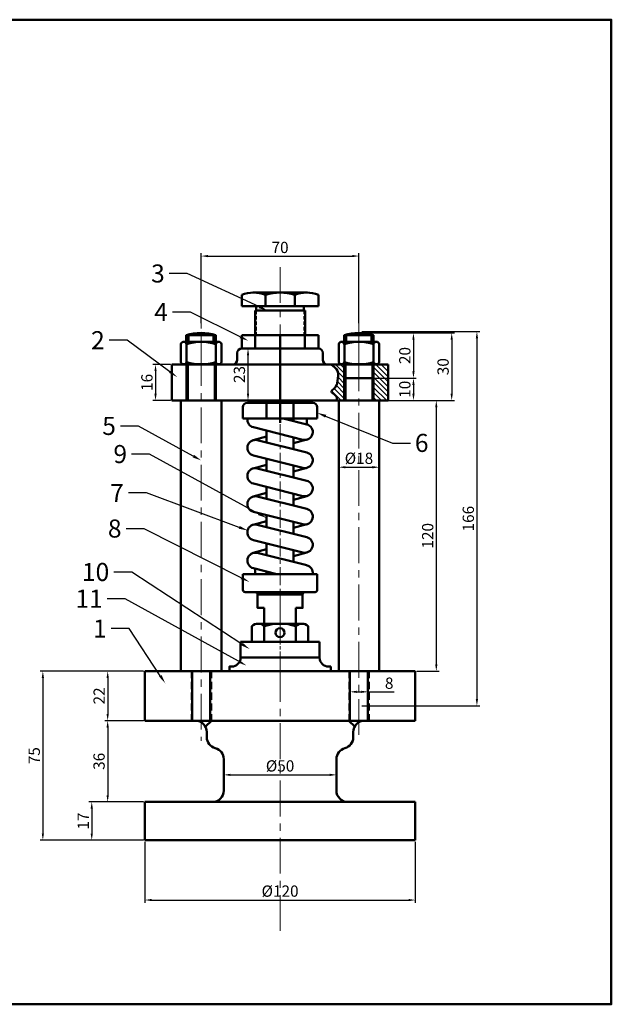
# Model space of a CAD drawing. Units: millimetres. Extents: x -656 to 85, y 134 to 571.
# Tile 5 of 5: x -178 to 85, y 134 to 571. Entities that reach past the tile are written whole.
import ezdxf
from ezdxf import colors
from ezdxf.entities.mleader import LeaderData, LeaderLine
from ezdxf.math import Vec2, Vec3

# ---------------------------------------------------------------- set-up
doc = ezdxf.new("R2010")
doc.units = ezdxf.units.MM
doc.header["$LTSCALE"] = 0.5
doc.linetypes.add('CENTER', pattern=[50.8, 31.75, -6.35, 6.35, -6.35])
doc.linetypes.add('HIDDEN', pattern=[9.525, 6.35, -3.175])
for name, color, linetype, lineweight in [('M-CNTR', 1, 'CENTER', 18), ('M-DIMS', 2, 'Continuous', 25), ('M-HATC', 8, 'Continuous', 18), ('M-HIDN', 3, 'HIDDEN', 25), ('M-OUTL', 7, 'Continuous', 50), ('M-TEXT', 7, 'Continuous', 25), ('M-TTLB', 7, 'Continuous', 50)]:
    doc.layers.add(name, color=color, linetype=linetype, lineweight=lineweight)
doc.styles.get("Standard").update_dxf_attribs({"font": 'arial.ttf'})
doc.dimstyles.new('ISO-25', dxfattribs={"dimtxt": 5, "dimasz": 3, "dimexe": 1.25, "dimexo": 0.625, "dimtad": 1, "dimtoh": 1, "dimdec": 0, "dimtxsty": 'Standard', "dimcen": 2.5, "dimadec": 0, "dimazin": 0, "dimtfac": 1, "dimtdec": 0, "dimtofl": 0, "dimtmove": 0, "dimatfit": 3, "dimfxl": 1, "dimarcsym": 0})

# ---------------------------------------------------------------- blocks, each defined once
blk = doc.blocks.new('*U82')
at = {"layer": 'M-CNTR', "color": 0, "transparency": 16777216}
blk.add_line((0, -16.59), (0, 25.52), dxfattribs=at)
blk = doc.blocks.new('*U83')
at = {"layer": 'M-CNTR', "color": 0, "transparency": 16777216}
blk.add_line((0, -7.5), (0, 12.59), dxfattribs=at)
blk = doc.blocks.new('*U84')
at = {"layer": 'M-CNTR', "color": 0, "transparency": 16777216}
blk.add_line((0, -7.5), (0, 12.59), dxfattribs=at)
blk = doc.blocks.new('*D85')
at = {"layer": 'Defpoints', "color": 0, "ltscale": 0.5, "transparency": 16777216}
for p in [(-122.34, 207.21), (-2.34, 207.21), (-2.34, 180.72)]:
    blk.add_point(p, dxfattribs=at)
at = {"layer": 'M-DIMS', "color": 0, "lineweight": -2, "ltscale": 0.5, "transparency": 16777216}
for p, q in [((-122.34, 206.59), (-122.34, 179.47)), ((-2.34, 206.59), (-2.34, 179.47)), ((-119.34, 180.72), (-5.34, 180.72))]:
    blk.add_line(p, q, dxfattribs=at)
at = {"layer": 'M-DIMS', "color": 0, "ltscale": 0.5, "transparency": 16777216}
for points in [[(-119.34, 181.22), (-119.34, 180.22), (-122.34, 180.72)], [(-5.34, 181.22), (-5.34, 180.22), (-2.34, 180.72)]]:
    blk.add_solid(points, dxfattribs=at)
at = {"layer": 'M-DIMS', "color": 0, "ltscale": 0.5, "transparency": 16777216, "insert": (-62.34, 184.03), "char_height": 5, "attachment_point": 5}
blk.add_mtext('%%C120', dxfattribs=at)
blk = doc.blocks.new('*D86')
at = {"layer": 'Defpoints', "color": 0, "ltscale": 0.5, "transparency": 16777216}
for p in [(-122.34, 282.21), (-167.59, 207.21), (-122.34, 207.21)]:
    blk.add_point(p, dxfattribs=at)
at = {"layer": 'M-DIMS', "color": 0, "lineweight": -2, "ltscale": 0.5, "transparency": 16777216}
for p, q in [((-122.96, 282.21), (-168.84, 282.21)), ((-167.59, 279.21), (-167.59, 210.21)), ((-122.96, 207.21), (-168.84, 207.21))]:
    blk.add_line(p, q, dxfattribs=at)
at = {"layer": 'M-DIMS', "color": 0, "ltscale": 0.5, "transparency": 16777216}
for points in [[(-168.09, 279.21), (-167.09, 279.21), (-167.59, 282.21)], [(-168.09, 210.21), (-167.09, 210.21), (-167.59, 207.21)]]:
    blk.add_solid(points, dxfattribs=at)
at = {"layer": 'M-DIMS', "color": 0, "ltscale": 0.5, "transparency": 16777216, "insert": (-170.76, 244.71), "char_height": 5, "attachment_point": 5, "rotation": 90}
blk.add_mtext('75', dxfattribs=at)
blk = doc.blocks.new('*D87')
at = {"layer": 'Defpoints', "color": 0, "ltscale": 0.5, "transparency": 16777216}
for p in [(-122.34, 282.21), (-138.83, 260.21), (-122.34, 260.21)]:
    blk.add_point(p, dxfattribs=at)
at = {"layer": 'M-DIMS', "color": 0, "lineweight": -2, "ltscale": 0.5, "transparency": 16777216}
for p, q in [((-122.96, 282.21), (-140.08, 282.21)), ((-138.83, 279.21), (-138.83, 263.21)), ((-122.96, 260.21), (-140.08, 260.21))]:
    blk.add_line(p, q, dxfattribs=at)
at = {"layer": 'M-DIMS', "color": 0, "ltscale": 0.5, "transparency": 16777216}
for points in [[(-139.33, 279.21), (-138.33, 279.21), (-138.83, 282.21)], [(-139.33, 263.21), (-138.33, 263.21), (-138.83, 260.21)]]:
    blk.add_solid(points, dxfattribs=at)
at = {"layer": 'M-DIMS', "color": 0, "ltscale": 0.5, "transparency": 16777216, "insert": (-141.97, 271.21), "char_height": 5, "attachment_point": 5, "rotation": 90}
blk.add_mtext('22', dxfattribs=at)
blk = doc.blocks.new('*D88')
at = {"layer": 'Defpoints', "color": 0, "ltscale": 0.5, "transparency": 16777216}
for p in [(-122.34, 224.21), (-145.9, 207.21), (-122.34, 207.21)]:
    blk.add_point(p, dxfattribs=at)
at = {"layer": 'M-DIMS', "color": 0, "lineweight": -2, "ltscale": 0.5, "transparency": 16777216}
for p, q in [((-122.96, 224.21), (-147.15, 224.21)), ((-145.9, 221.21), (-145.9, 210.21)), ((-122.96, 207.21), (-147.15, 207.21))]:
    blk.add_line(p, q, dxfattribs=at)
at = {"layer": 'M-DIMS', "color": 0, "ltscale": 0.5, "transparency": 16777216}
for points in [[(-146.4, 221.21), (-145.4, 221.21), (-145.9, 224.21)], [(-146.4, 210.21), (-145.4, 210.21), (-145.9, 207.21)]]:
    blk.add_solid(points, dxfattribs=at)
at = {"layer": 'M-DIMS', "color": 0, "ltscale": 0.5, "transparency": 16777216, "insert": (-149.04, 215.71), "char_height": 5, "attachment_point": 5, "rotation": 90}
blk.add_mtext('17', dxfattribs=at)
blk = doc.blocks.new('*D89')
at = {"layer": 'Defpoints', "color": 0, "ltscale": 0.5, "transparency": 16777216}
for p in [(-122.34, 260.21), (-138.83, 224.21), (-122.34, 224.21)]:
    blk.add_point(p, dxfattribs=at)
at = {"layer": 'M-DIMS', "color": 0, "lineweight": -2, "ltscale": 0.5, "transparency": 16777216}
for p, q in [((-122.96, 260.21), (-140.08, 260.21)), ((-138.83, 257.21), (-138.83, 227.21)), ((-122.96, 224.21), (-140.08, 224.21))]:
    blk.add_line(p, q, dxfattribs=at)
at = {"layer": 'M-DIMS', "color": 0, "ltscale": 0.5, "transparency": 16777216}
for points in [[(-139.33, 257.21), (-138.33, 257.21), (-138.83, 260.21)], [(-139.33, 227.21), (-138.33, 227.21), (-138.83, 224.21)]]:
    blk.add_solid(points, dxfattribs=at)
at = {"layer": 'M-DIMS', "color": 0, "ltscale": 0.5, "transparency": 16777216, "insert": (-142.01, 242.21), "char_height": 5, "attachment_point": 5, "rotation": 90}
blk.add_mtext('36', dxfattribs=at)
blk = doc.blocks.new('*D90')
at = {"layer": 'Defpoints', "color": 0, "ltscale": 0.5, "transparency": 16777216}
for p in [(-87.34, 236.21), (-37.34, 236.21), (-37.34, 236.21)]:
    blk.add_point(p, dxfattribs=at)
at = {"layer": 'M-DIMS', "color": 0, "lineweight": -2, "ltscale": 0.5, "transparency": 16777216}
for p, q in [((-87.34, 236.84), (-87.34, 237.46)), ((-84.34, 236.21), (-40.34, 236.21)), ((-37.34, 236.84), (-37.34, 237.46))]:
    blk.add_line(p, q, dxfattribs=at)
at = {"layer": 'M-DIMS', "color": 0, "ltscale": 0.5, "transparency": 16777216}
for points in [[(-84.34, 236.71), (-84.34, 235.71), (-87.34, 236.21)], [(-40.34, 236.71), (-40.34, 235.71), (-37.34, 236.21)]]:
    blk.add_solid(points, dxfattribs=at)
at = {"layer": 'M-DIMS', "color": 0, "ltscale": 0.5, "transparency": 16777216, "insert": (-62.34, 239.53), "char_height": 5, "attachment_point": 5}
blk.add_mtext('%%C50', dxfattribs=at)
blk = doc.blocks.new('*D91')
at = {"layer": 'Defpoints', "color": 0, "ltscale": 0.5, "transparency": 16777216}
for p in [(-31.34, 271.21), (-23.34, 273.03), (-23.34, 271.21)]:
    blk.add_point(p, dxfattribs=at)
at = {"layer": 'M-DIMS', "color": 0, "lineweight": -2, "ltscale": 0.5, "transparency": 16777216}
for p, q in [((-31.34, 271.84), (-31.34, 274.28)), ((-28.34, 273.03), (-26.34, 273.03)), ((-23.34, 271.84), (-23.34, 274.28)), ((-23.34, 273.03), (-11.66, 273.03))]:
    blk.add_line(p, q, dxfattribs=at)
at = {"layer": 'M-DIMS', "color": 0, "ltscale": 0.5, "transparency": 16777216}
for points in [[(-28.34, 273.53), (-28.34, 272.53), (-31.34, 273.03)], [(-26.34, 273.53), (-26.34, 272.53), (-23.34, 273.03)]]:
    blk.add_solid(points, dxfattribs=at)
at = {"layer": 'M-DIMS', "color": 0, "ltscale": 0.5, "transparency": 16777216, "insert": (-13.93, 276.21), "char_height": 5, "attachment_point": 5}
blk.add_mtext('8', dxfattribs=at)
blk = doc.blocks.new('*D92')
at = {"layer": 'Defpoints', "color": 0, "ltscale": 0.5, "transparency": 16777216}
for p in [(-26.71, 432.8), (-26.71, 266.8), (25, 266.8)]:
    blk.add_point(p, dxfattribs=at)
at = {"layer": 'M-DIMS', "color": 0, "lineweight": -2, "ltscale": 0.5, "transparency": 16777216}
for p, q in [((-26.09, 432.8), (26.25, 432.8)), ((25, 429.8), (25, 269.8)), ((-26.09, 266.8), (26.25, 266.8))]:
    blk.add_line(p, q, dxfattribs=at)
at = {"layer": 'M-DIMS', "color": 0, "ltscale": 0.5, "transparency": 16777216}
for points in [[(24.5, 429.8), (25.5, 429.8), (25, 432.8)], [(24.5, 269.8), (25.5, 269.8), (25, 266.8)]]:
    blk.add_solid(points, dxfattribs=at)
at = {"layer": 'M-DIMS', "color": 0, "ltscale": 0.5, "transparency": 16777216, "insert": (21.82, 349.8), "char_height": 5, "attachment_point": 5, "rotation": 90}
blk.add_mtext('166', dxfattribs=at)
blk = doc.blocks.new('*D93')
at = {"layer": 'Defpoints', "color": 0, "ltscale": 0.5, "transparency": 16777216}
for p in [(-27.4, 432.12), (-27.34, 402.21), (13.81, 402.21)]:
    blk.add_point(p, dxfattribs=at)
at = {"layer": 'M-DIMS', "color": 0, "lineweight": -2, "ltscale": 0.5, "transparency": 16777216}
for p, q in [((-26.77, 432.12), (15.06, 432.12)), ((13.81, 429.12), (13.81, 405.21)), ((-26.71, 402.21), (15.06, 402.21))]:
    blk.add_line(p, q, dxfattribs=at)
at = {"layer": 'M-DIMS', "color": 0, "ltscale": 0.5, "transparency": 16777216}
for points in [[(13.31, 429.12), (14.31, 429.12), (13.81, 432.12)], [(13.31, 405.21), (14.31, 405.21), (13.81, 402.21)]]:
    blk.add_solid(points, dxfattribs=at)
at = {"layer": 'M-DIMS', "color": 0, "ltscale": 0.5, "transparency": 16777216, "insert": (10.63, 417.17), "char_height": 5, "attachment_point": 5, "rotation": 90}
blk.add_mtext('30', dxfattribs=at)
blk = doc.blocks.new('*D94')
at = {"layer": 'Defpoints', "color": 0, "ltscale": 0.5, "transparency": 16777216}
for p in [(-27.34, 432.12), (-27.34, 412.12), (-3.16, 412.12)]:
    blk.add_point(p, dxfattribs=at)
at = {"layer": 'M-DIMS', "color": 0, "lineweight": -2, "ltscale": 0.5, "transparency": 16777216}
for p, q in [((-26.71, 432.12), (-1.91, 432.12)), ((-3.16, 429.12), (-3.16, 415.12)), ((-26.71, 412.12), (-1.91, 412.12))]:
    blk.add_line(p, q, dxfattribs=at)
at = {"layer": 'M-DIMS', "color": 0, "ltscale": 0.5, "transparency": 16777216}
for points in [[(-3.66, 429.12), (-2.66, 429.12), (-3.16, 432.12)], [(-3.66, 415.12), (-2.66, 415.12), (-3.16, 412.12)]]:
    blk.add_solid(points, dxfattribs=at)
at = {"layer": 'M-DIMS', "color": 0, "ltscale": 0.5, "transparency": 16777216, "insert": (-6.34, 422.12), "char_height": 5, "attachment_point": 5, "rotation": 90}
blk.add_mtext('20', dxfattribs=at)
blk = doc.blocks.new('*D95')
at = {"layer": 'Defpoints', "color": 0, "ltscale": 0.5, "transparency": 16777216}
for p in [(-11.41, 412.12), (-11.41, 402.21), (-3.16, 402.21)]:
    blk.add_point(p, dxfattribs=at)
at = {"layer": 'M-DIMS', "color": 0, "lineweight": -2, "ltscale": 0.5, "transparency": 16777216}
for p, q in [((-10.78, 412.12), (-1.91, 412.12)), ((-3.16, 409.12), (-3.16, 405.21)), ((-10.78, 402.21), (-1.91, 402.21))]:
    blk.add_line(p, q, dxfattribs=at)
at = {"layer": 'M-DIMS', "color": 0, "ltscale": 0.5, "transparency": 16777216}
for points in [[(-3.66, 409.12), (-2.66, 409.12), (-3.16, 412.12)], [(-3.66, 405.21), (-2.66, 405.21), (-3.16, 402.21)]]:
    blk.add_solid(points, dxfattribs=at)
at = {"layer": 'M-DIMS', "color": 0, "ltscale": 0.5, "transparency": 16777216, "insert": (-6.34, 407.17), "char_height": 5, "attachment_point": 5, "rotation": 90}
blk.add_mtext('10', dxfattribs=at)
blk = doc.blocks.new('*D96')
at = {"layer": 'Defpoints', "color": 0, "ltscale": 0.5, "transparency": 16777216}
for p in [(-36.34, 372.6), (-18.34, 372.6), (-18.34, 372.6)]:
    blk.add_point(p, dxfattribs=at)
at = {"layer": 'M-DIMS', "color": 0, "lineweight": -2, "ltscale": 0.5, "transparency": 16777216}
for p, q in [((-36.34, 373.23), (-36.34, 373.85)), ((-33.34, 372.6), (-21.34, 372.6)), ((-18.34, 373.23), (-18.34, 373.85))]:
    blk.add_line(p, q, dxfattribs=at)
at = {"layer": 'M-DIMS', "color": 0, "ltscale": 0.5, "transparency": 16777216}
for points in [[(-33.34, 373.1), (-33.34, 372.1), (-36.34, 372.6)], [(-21.34, 373.1), (-21.34, 372.1), (-18.34, 372.6)]]:
    blk.add_solid(points, dxfattribs=at)
at = {"layer": 'M-DIMS', "color": 0, "ltscale": 0.5, "transparency": 16777216, "insert": (-27.34, 375.92), "char_height": 5, "attachment_point": 5}
blk.add_mtext('%%C18', dxfattribs=at)
blk = doc.blocks.new('*D97')
at = {"layer": 'Defpoints', "color": 0, "ltscale": 0.5, "transparency": 16777216}
for p in [(1.86, 402.21), (-2.34, 282.21), (6.97, 282.21)]:
    blk.add_point(p, dxfattribs=at)
at = {"layer": 'M-DIMS', "color": 0, "lineweight": -2, "ltscale": 0.5, "transparency": 16777216}
for p, q in [((2.49, 402.21), (8.22, 402.21)), ((6.97, 399.21), (6.97, 285.21)), ((-1.71, 282.21), (8.22, 282.21))]:
    blk.add_line(p, q, dxfattribs=at)
at = {"layer": 'M-DIMS', "color": 0, "ltscale": 0.5, "transparency": 16777216}
for points in [[(6.47, 399.21), (7.47, 399.21), (6.97, 402.21)], [(6.47, 285.21), (7.47, 285.21), (6.97, 282.21)]]:
    blk.add_solid(points, dxfattribs=at)
at = {"layer": 'M-DIMS', "color": 0, "ltscale": 0.5, "transparency": 16777216, "insert": (3.8, 342.21), "char_height": 5, "attachment_point": 5, "rotation": 90}
blk.add_mtext('120', dxfattribs=at)
blk = doc.blocks.new('*D98')
at = {"layer": 'Defpoints', "color": 0, "ltscale": 0.5, "transparency": 16777216}
for p in [(-110.34, 418.21), (-117.6, 402.21), (-110.34, 402.21)]:
    blk.add_point(p, dxfattribs=at)
at = {"layer": 'M-DIMS', "color": 0, "lineweight": -2, "ltscale": 0.5, "transparency": 16777216}
for p, q in [((-110.96, 418.21), (-118.85, 418.21)), ((-117.6, 415.21), (-117.6, 405.21)), ((-110.96, 402.21), (-118.85, 402.21))]:
    blk.add_line(p, q, dxfattribs=at)
at = {"layer": 'M-DIMS', "color": 0, "ltscale": 0.5, "transparency": 16777216}
for points in [[(-118.1, 415.21), (-117.1, 415.21), (-117.6, 418.21)], [(-118.1, 405.21), (-117.1, 405.21), (-117.6, 402.21)]]:
    blk.add_solid(points, dxfattribs=at)
at = {"layer": 'M-DIMS', "color": 0, "ltscale": 0.5, "transparency": 16777216, "insert": (-120.78, 410.21), "char_height": 5, "attachment_point": 5, "rotation": 90}
blk.add_mtext('16', dxfattribs=at)
blk = doc.blocks.new('*D99')
at = {"layer": 'Defpoints', "color": 0, "ltscale": 0.5, "transparency": 16777216}
for p in [(-27.34, 466.22), (-97.34, 435.8), (-27.34, 435.8)]:
    blk.add_point(p, dxfattribs=at)
at = {"layer": 'M-DIMS', "color": 0, "lineweight": -2, "ltscale": 0.5, "transparency": 16777216}
for p, q in [((-97.34, 436.43), (-97.34, 467.47)), ((-27.34, 436.43), (-27.34, 467.47)), ((-94.34, 466.22), (-30.34, 466.22))]:
    blk.add_line(p, q, dxfattribs=at)
at = {"layer": 'M-DIMS', "color": 0, "ltscale": 0.5, "transparency": 16777216}
for points in [[(-94.34, 466.72), (-94.34, 465.72), (-97.34, 466.22)], [(-30.34, 466.72), (-30.34, 465.72), (-27.34, 466.22)]]:
    blk.add_solid(points, dxfattribs=at)
at = {"layer": 'M-DIMS', "color": 0, "ltscale": 0.5, "transparency": 16777216, "insert": (-62.34, 469.4), "char_height": 5, "attachment_point": 5}
blk.add_mtext('70', dxfattribs=at)
blk = doc.blocks.new('*D100')
at = {"layer": 'Defpoints', "color": 0, "ltscale": 0.5, "transparency": 16777216}
for p in [(-76.68, 425.21), (-76.56, 425.21), (-76.68, 402.21)]:
    blk.add_point(p, dxfattribs=at)
at = {"layer": 'M-DIMS', "color": 0, "lineweight": -2, "ltscale": 0.5, "transparency": 16777216}
for p, q in [((-76.06, 425.21), (-75.31, 425.21)), ((-76.56, 405.21), (-76.56, 422.21)), ((-76.06, 402.21), (-75.31, 402.21))]:
    blk.add_line(p, q, dxfattribs=at)
at = {"layer": 'M-DIMS', "color": 0, "ltscale": 0.5, "transparency": 16777216}
for points in [[(-77.06, 422.21), (-76.06, 422.21), (-76.56, 425.21)], [(-77.06, 405.21), (-76.06, 405.21), (-76.56, 402.21)]]:
    blk.add_solid(points, dxfattribs=at)
at = {"layer": 'M-DIMS', "color": 0, "ltscale": 0.5, "transparency": 16777216, "insert": (-79.74, 413.71), "char_height": 5, "attachment_point": 5, "rotation": 90}
blk.add_mtext('23', dxfattribs=at)
blk = doc.blocks.new('NUT-HEX-LOCK')
at = {"ltscale": 0.5}
for p, q in [((38.72, -408.22), (38.72, -405.22)), ((51.84, -405.22), (38.72, -405.22)), ((51.84, -408.22), (51.84, -405.22)), ((36.34, -409.22), (36.34, -417.22)), ((38.84, -409.22), (38.84, -417.22)), ((51.84, -417.22), (51.84, -409.22)), ((54.34, -417.22), (54.34, -409.22))]:
    blk.add_line(p, q, dxfattribs=at)
for centre, radius, start, end in [((45.28, -428.53), 24.22, 74.2897, 105.7103), ((37.59, -409.5), 1.28, 12.6787, 167.3213), ((45.34, -429.84), 21.62, 72.5077, 107.4923), ((53.09, -409.5), 1.28, 12.6782, 167.3218), ((37.59, -416.93), 1.28, 192.6787, 347.3213), ((45.34, -396.59), 21.62, 252.5077, 287.4923), ((53.09, -416.93), 1.28, 192.6782, 347.3218)]:
    blk.add_arc(centre, radius, start, end, dxfattribs=at)
blk = doc.blocks.new('STUD-ROD')
at = {"ltscale": 0.5}
for p, q in [((0, 120), (0, 0)), ((18, 120), (0, 120)), ((18, 0), (18, 120)), ((0, 0), (18, 0))]:
    blk.add_line(p, q, dxfattribs=at)

msp = doc.modelspace()

# ---------------------------------------------------------------- hatches: boundary and pattern name
at = {"layer": 'M-HATC', "ltscale": 0.5}
h = msp.add_hatch(dxfattribs=at)
h.set_pattern_fill('ANSI31', color=256, scale=0.5, angle=90)
h.set_pattern_definition([(135, (-1832.0751, -452.3756), (-1.122532, -1.122532), [])])
h.paths.add_polyline_path([(-14.34, 418.21), (-20.84, 418.21), (-20.84, 402.21), (-18.34, 402.21), (-14.34, 402.21)])
edge = h.paths.add_edge_path()
edge.add_line((-33.84, 418.21), (-35.1, 418.21))
edge.add_line((-35.1, 418.21), (-39.78, 418.21))
edge.add_spline(control_points=[(-39.78, 418.21), (-38.56, 417.35), (-36.05, 415.56), (-36.85, 411.09), (-37.28, 407.9), (-40.74, 405.9), (-37.02, 404.71), (-37.01, 402.69), (-37.37, 402.21)], knot_values=[0, 0, 0, 0, 4.136966, 8.535604, 12.069689, 14.056123, 17.152579, 18.950395, 18.950395, 18.950395, 18.950395], degree=3, periodic=0)
edge.add_line((-37.37, 402.21), (-33.84, 402.21))
edge.add_line((-33.84, 402.21), (-33.84, 418.21))

# ---------------------------------------------------------------- linework, layer by layer
at = {"layer": 'M-CNTR'}
for p, q in [((-97.34, 449.93), (-97.34, 251.34)), ((-27.34, 447.57), (-27.34, 252.71)), ((-62.34, 167.01), (-62.34, 307.88))]:
    msp.add_line(p, q, dxfattribs=at)
at = {"layer": 'M-CNTR', "ltscale": 0.5}
msp.add_line((-62.34, 282.21), (-62.34, 399.02), dxfattribs=at)
at = {"layer": 'M-HIDN', "ltscale": 0.5}
for p, q in [((-72.94, 442.02), (-72.94, 431.21)), ((-51.74, 442.02), (-51.74, 431.21))]:
    msp.add_line(p, q, dxfattribs=at)
at = {"layer": 'M-HIDN'}
for p, q in [((-101.84, 282.21), (-101.84, 260.21)), ((-92.84, 282.21), (-92.84, 260.21)), ((-31.84, 282.21), (-31.84, 260.21)), ((-22.84, 282.21), (-22.84, 260.21))]:
    msp.add_line(p, q, dxfattribs=at)
at = {"layer": 'M-OUTL', "ltscale": 0.5}
for p, q in [((-74.48, 450.02), (-50.24, 450.02)), ((-79.34, 444.02), (-79.34, 449.02)), ((-68.84, 444.02), (-68.84, 449.02)), ((-55.84, 444.02), (-55.84, 449.02)), ((-45.34, 449.02), (-45.34, 444.02)), ((-51.74, 444.02), (-79.34, 444.02)), ((-73.44, 431.21), (-73.44, 442.02)), ((-72.94, 442.02), (-73.44, 442.02)), ((-72.94, 444.02), (-72.94, 442.2)), ((-72.94, 442.02), (-72.94, 442.2)), ((-72.94, 442.02), (-51.74, 442.02)), ((-45.34, 444.02), (-51.74, 444.02)), ((-51.74, 444.02), (-51.74, 442.02)), ((-51.24, 442.02), (-51.74, 442.02)), ((-51.24, 431.21), (-51.24, 442.02)), ((-89.58, 428.21), (-105.1, 428.21)), ((-102.95, 428.21), (-102.95, 431.21)), ((-91.84, 428.21), (-91.84, 431.21)), ((-79.34, 431.21), (-45.34, 431.21)), ((-79.34, 425.21), (-79.34, 431.21)), ((-73.34, 425.21), (-73.34, 431.21)), ((-62.34, 431.21), (-62.34, 425.21)), ((-51.34, 425.21), (-51.34, 431.21)), ((-45.34, 431.21), (-45.34, 425.21)), ((-19.58, 428.21), (-35.1, 428.21)), ((-32.95, 428.21), (-32.95, 431.21)), ((-21.84, 428.21), (-21.84, 431.21)), ((-79.34, 425.21), (-45.34, 425.21)), ((-45.34, 425.21), (-79.34, 425.21)), ((-62.34, 425.21), (-62.34, 402.21)), ((-62.34, 402.21), (-62.34, 425.21)), ((-81.34, 423.21), (-81.34, 420.21)), ((-43.34, 423.21), (-43.34, 420.21)), ((-110.34, 418.21), (-41.34, 418.21)), ((-110.34, 418.21), (-110.34, 402.21)), ((-105.1, 418.21), (-89.58, 418.21)), ((-103.84, 418.21), (-103.84, 402.21)), ((-103.34, 418.21), (-103.34, 402.21)), ((-91.34, 418.21), (-91.34, 402.21)), ((-90.84, 418.21), (-90.84, 402.21)), ((-62.34, 402.21), (-62.34, 418.21)), ((-41.34, 418.21), (-14.34, 418.21)), ((-35.1, 418.21), (-19.58, 418.21)), ((-33.84, 418.21), (-33.84, 402.21)), ((-33.34, 418.21), (-33.34, 402.21)), ((-21.34, 418.21), (-21.34, 402.21)), ((-20.84, 418.21), (-20.84, 402.21)), ((-14.34, 402.21), (-14.34, 418.21)), ((-21.34, 412.12), (-33.34, 412.12)), ((-110.34, 402.21), (-14.34, 402.21)), ((-72.87, 401.85), (-51.71, 401.85)), ((-68.34, 402.21), (-68.34, 394.21)), ((-62.34, 392.28), (-62.34, 405.21)), ((-56.34, 393.07), (-56.34, 402.21)), ((-78.84, 399.21), (-78.84, 394.21)), ((-76.84, 401.21), (-68.34, 401.21)), ((-68.34, 397.21), (-68.34, 401.21)), ((-68.34, 401.21), (-50.34, 401.21)), ((-56.34, 397.21), (-56.34, 401.21)), ((-50.34, 401.21), (-47.84, 401.21)), ((-45.84, 394.21), (-45.84, 399.21)), ((-78.84, 394.21), (-76.8, 394.21)), ((-76.8, 394.21), (-45.84, 394.21)), ((-60.91, 394.21), (-50.49, 391.61)), ((-50.49, 391.61), (-50.49, 394.21)), ((-74.19, 390.32), (-52.19, 384.82)), ((-68.34, 388.86), (-68.34, 383.57)), ((-74.26, 384.59), (-68.34, 386.21)), ((-72.49, 384.61), (-50.49, 379.11)), ((-56.34, 380.57), (-56.34, 385.86)), ((-56.34, 383.21), (-50.41, 384.84)), ((-74.19, 377.82), (-52.19, 372.32)), ((-68.34, 376.36), (-68.34, 371.07)), ((-74.26, 372.09), (-68.34, 373.71)), ((-72.49, 372.11), (-50.49, 366.61)), ((-56.34, 368.07), (-56.34, 373.36)), ((-56.34, 370.71), (-50.41, 372.34)), ((-74.19, 365.32), (-52.19, 359.82)), ((-68.34, 363.86), (-68.34, 358.57)), ((-74.26, 359.59), (-68.34, 361.21)), ((-72.49, 359.61), (-50.49, 354.11)), ((-56.34, 355.57), (-56.34, 360.86)), ((-56.34, 358.21), (-50.41, 359.84)), ((-74.19, 352.82), (-52.19, 347.32)), ((-68.34, 351.36), (-68.34, 346.07)), ((-74.26, 347.09), (-68.34, 348.71)), ((-72.49, 347.11), (-50.49, 341.61)), ((-56.34, 343.07), (-56.34, 348.36)), ((-56.34, 345.71), (-50.41, 347.34)), ((-74.26, 334.59), (-68.34, 336.21)), ((-74.19, 340.32), (-52.19, 334.82)), ((-68.34, 338.86), (-68.34, 333.57)), ((-72.49, 334.61), (-50.49, 329.11)), ((-56.34, 330.57), (-56.34, 335.86)), ((-56.34, 333.21), (-50.41, 334.84)), ((-74.19, 327.82), (-63.77, 325.21)), ((-73.34, 327.61), (-73.34, 325.21)), ((-78.84, 325.21), (-68.34, 325.21)), ((-78.84, 318.21), (-78.84, 325.21)), ((-76.84, 325.21), (-56.34, 325.21)), ((-68.34, 326.36), (-68.34, 325.21)), ((-56.34, 325.21), (-45.84, 325.21)), ((-56.34, 325.21), (-47.84, 325.21)), ((-45.84, 325.21), (-45.84, 318.21)), ((-51.34, 317.21), (-77.84, 317.21)), ((-68.34, 317.21), (-68.34, 316.21)), ((-68.34, 316.21), (-56.34, 316.21)), ((-60.34, 316.21), (-64.34, 316.21)), ((-56.34, 316.21), (-56.34, 317.21)), ((-46.84, 317.21), (-51.34, 317.21)), ((-69.34, 310.21), (-69.34, 303.21)), ((-55.34, 303.21), (-55.34, 310.21)), ((-74.84, 295.21), (-74.84, 302.21)), ((-72.09, 303.21), (-52.59, 303.21)), ((-69.34, 302.21), (-69.34, 295.21)), ((-55.34, 295.21), (-55.34, 302.21)), ((-49.84, 302.21), (-49.84, 295.21)), ((-79.84, 288.21), (-79.84, 295.21)), ((-79.84, 295.21), (-44.84, 295.21)), ((-69.34, 295.21), (-69.34, 295.36)), ((-44.84, 295.21), (-44.84, 288.21)), ((-44.84, 288.21), (-79.84, 288.21)), ((-31.84, 260.21), (-22.84, 260.21)), ((-31.84, 260.21), (-29.23, 257.61))]:
    msp.add_line(p, q, dxfattribs=at)
at = {"layer": 'M-OUTL'}
for p, q in [((-122.34, 282.21), (-31.84, 282.21)), ((-122.34, 282.21), (-122.34, 260.21)), ((-101.34, 282.21), (-101.34, 260.21)), ((-93.34, 282.21), (-93.34, 260.21)), ((-42.34, 282.21), (-2.34, 282.21)), ((-42.34, 282.21), (-27.34, 282.21)), ((-31.34, 282.21), (-31.34, 260.21)), ((-23.34, 282.21), (-23.34, 260.21)), ((-2.34, 260.21), (-2.34, 282.21)), ((-122.34, 260.21), (-97.34, 260.21)), ((-101.84, 260.21), (-31.84, 260.21)), ((-92.84, 260.21), (-95.45, 257.61)), ((-24.84, 260.21), (-2.34, 260.21)), ((-94.84, 252.9), (-94.84, 255.21)), ((-29.84, 252.9), (-29.84, 255.21)), ((-87.34, 229.21), (-87.34, 243.21)), ((-37.34, 229.21), (-37.34, 243.21)), ((-2.34, 224.21), (-122.34, 224.21)), ((-122.34, 224.21), (-122.34, 207.21)), ((-2.34, 224.21), (-32.34, 224.21)), ((-2.34, 207.21), (-2.34, 224.21)), ((-122.34, 207.21), (-2.34, 207.21))]:
    msp.add_line(p, q, dxfattribs=at)
at = {"layer": 'M-OUTL', "ltscale": 0.5}
for points in [[(-52.34, 316.21), (-72.34, 316.21)], [(-72.34, 316.21), (-72.34, 310.21), (-69.34, 310.21)], [(-55.34, 310.21), (-52.34, 310.21), (-52.34, 316.21)]]:
    msp.add_lwpolyline(points, dxfattribs=at)
msp.add_lwpolyline([(-39.84, 284.21), (-39.84, 282.21), (-84.84, 282.21), (-84.84, 284.21), (-83.84, 284.21, 0.414214), (-79.84, 288.21), (-44.84, 288.21, 0.414214), (-40.84, 284.21)], format="xyb", close=True, dxfattribs=at)
msp.add_circle((-62.34, 299.21), 2, dxfattribs=at)
msp.add_circle((-62.34, 299.21), 2, dxfattribs=at)
for centre, radius, start, end in [((-74.09, 435.81), 14.21, 68.3188, 111.6812), ((-62.34, 428.39), 21.63, 72.5077, 107.4923), ((-50.59, 435.8), 14.23, 68.3433, 111.6567), ((-79.34, 423.21), 2, 90, 180), ((-45.34, 423.21), 2, 0, 90), ((-83.34, 420.21), 2, 270, 0), ((-41.34, 420.21), 2, 180, 270), ((-74.34, 403.21), 2, 270, 330), ((-50.34, 403.21), 2, 210, 270), ((-76.84, 399.21), 2, 90, 180), ((-47.84, 399.21), 2, 0, 90), ((-73.34, 393.71), 3.5, 171.7868, 255.9638), ((-51.34, 388.21), 3.5, 255.9638, 75.9638), ((-73.34, 381.21), 3.5, 75.9638, 255.9638), ((-51.34, 375.71), 3.5, 255.9638, 75.9638), ((-73.34, 368.71), 3.5, 75.9638, 255.9638), ((-51.34, 363.21), 3.5, 255.9638, 75.9638), ((-73.34, 356.21), 3.5, 75.9638, 255.9638), ((-51.34, 350.71), 3.5, 255.9638, 75.9638), ((-73.34, 343.71), 3.5, 75.9638, 255.9638), ((-51.34, 338.21), 3.5, 255.9638, 75.9638), ((-73.34, 331.21), 3.5, 75.9638, 255.9638), ((-51.34, 325.71), 3.5, 351.7868, 75.9638), ((-77.84, 318.21), 1, 180, 270), ((-73.34, 316.21), 1, 0, 90), ((-51.34, 316.21), 1, 90, 180), ((-46.84, 318.21), 1, 270, 0), ((-72.09, 298.93), 4.28, 50.0338, 129.9662), ((-62.34, 278.21), 25, 73.7398, 106.2602), ((-52.59, 298.93), 4.28, 50.0338, 129.9662), ((-62.34, 288.21), 10, 134.427, 135.573)]:
    msp.add_arc(centre, radius, start, end, dxfattribs=at)
at = {"layer": 'M-OUTL'}
for centre, start, end in [((-99.84, 255.21), 0, 90), ((-24.84, 255.21), 90, 180), ((-89.84, 252.9), 180, 255.5225), ((-34.84, 252.9), 284.4775, 0), ((-92.34, 243.21), 0, 75.5225), ((-32.34, 243.21), 104.4775, 180), ((-92.34, 229.21), 270, 0), ((-32.34, 229.21), 180, 270)]:
    msp.add_arc(centre, 5, start, end, dxfattribs=at)
at = {"layer": 'M-OUTL', "ltscale": 0.5}
msp.add_open_spline([(-39.78, 418.21), (-38.56, 417.35), (-36.05, 415.56), (-36.85, 411.09), (-37.28, 407.9), (-40.74, 405.9), (-37.02, 404.71), (-37.01, 402.69), (-37.37, 402.21)], degree=3, knots=[0, 0, 0, 0, 4.136966, 8.535604, 12.069689, 14.056123, 17.152579, 18.950395, 18.950395, 18.950395, 18.950395], dxfattribs=at)
at = {"layer": 'M-TTLB', "ltscale": 0.5}
msp.add_lwpolyline([(-656.34, 571.01), (84.63, 571.01), (84.63, 134.49), (-656.34, 134.49)], close=True, dxfattribs=at)

# ---------------------------------------------------------------- block references
at = {"layer": 'M-CNTR'}
for name, p in [('*U82', (-62.34, 436.62)), ('*U84', (-97.34, 423.21)), ('*U83', (-27.34, 423.21))]:
    msp.add_blockref(name, p, dxfattribs=at)
at = {"layer": 'M-OUTL'}
for name, p in [('NUT-HEX-LOCK', (-142.67, 836.43)), ('NUT-HEX-LOCK', (-72.67, 836.43)), ('STUD-ROD', (-106.34, 282.21)), ('STUD-ROD', (-36.34, 282.21))]:
    msp.add_blockref(name, p, dxfattribs=at)

# ---------------------------------------------------------------- dimensions: what is measured, and where the dimension line sits
at = {"layer": 'M-DIMS', "ltscale": 0.5}
dim = msp.add_linear_dim(base=(-27.34, 466.22), p1=(-97.34, 435.8), p2=(-27.34, 435.8), dimstyle='ISO-25', override={"dimclrd": 0, "dimclre": 0, "dimclrt": 0}, dxfattribs=at)
dim.commit()
dim.dimension.update_dxf_attribs({"geometry": '*D99', "text_midpoint": (-62.34, 469.4)})
for base, p1, p2, picture, middle in [((25, 266.8), (-26.71, 432.8), (-26.71, 266.8), '*D92', (21.82, 349.8)), ((13.81, 402.21), (-27.4, 432.12), (-27.34, 402.21), '*D93', (10.63, 417.17)), ((-3.16, 412.12), (-27.34, 432.12), (-27.34, 412.12), '*D94', (-6.34, 422.12)), ((-76.56, 425.21), (-76.68, 402.21), (-76.68, 425.21), '*D100', (-79.74, 413.71)), ((-117.6, 402.21), (-110.34, 418.21), (-110.34, 402.21), '*D98', (-120.78, 410.21)), ((-3.16, 402.21), (-11.41, 412.12), (-11.41, 402.21), '*D95', (-6.34, 407.17)), ((6.97, 282.21), (1.86, 402.21), (-2.34, 282.21), '*D97', (3.8, 342.21)), ((-167.59, 207.21), (-122.34, 282.21), (-122.34, 207.21), '*D86', (-170.76, 244.71)), ((-138.83, 260.21), (-122.34, 282.21), (-122.34, 260.21), '*D87', (-141.97, 271.21)), ((-138.83, 224.21), (-122.34, 260.21), (-122.34, 224.21), '*D89', (-142.01, 242.21)), ((-145.9, 207.21), (-122.34, 224.21), (-122.34, 207.21), '*D88', (-149.04, 215.71))]:
    dim = msp.add_linear_dim(base=base, p1=p1, p2=p2, angle=90, dimstyle='ISO-25', override={"dimclrd": 0, "dimclre": 0, "dimclrt": 0}, dxfattribs=at)
    dim.commit()
    dim.dimension.update_dxf_attribs({"geometry": picture, "text_midpoint": middle})
for base, p1, p2, picture, middle in [((-18.34, 372.6), (-36.34, 372.6), (-18.34, 372.6), '*D96', (-27.34, 375.92)), ((-37.34, 236.21), (-87.34, 236.21), (-37.34, 236.21), '*D90', (-62.34, 239.53)), ((-2.34, 180.72), (-122.34, 207.21), (-2.34, 207.21), '*D85', (-62.34, 184.03))]:
    dim = msp.add_linear_dim(base=base, p1=p1, p2=p2, text='%%C<>', dimstyle='ISO-25', override={"dimclrd": 0, "dimclre": 0, "dimclrt": 0}, dxfattribs=at)
    dim.commit()
    dim.dimension.update_dxf_attribs({"geometry": picture, "text_midpoint": middle})
dim = msp.add_linear_dim(base=(-23.34, 273.03), p1=(-31.34, 271.21), p2=(-23.34, 271.21), dimstyle='ISO-25', override={"dimclrd": 0, "dimclre": 0, "dimclrt": 0}, dxfattribs=at)
dim.commit()
dim.dimension.update_dxf_attribs({"geometry": '*D91', "text_midpoint": (-13.93, 273.03), "dimtype": 160})

# ---------------------------------------------------------------- leaders
at = {"layer": 'M-TEXT', "ltscale": 0.5}
ml = msp.add_multileader_mtext('Standard', dxfattribs=at)
ml.set_content('3', color=256)
ml.set_leader_properties()
ml.build(insert=Vec2(0, 0))
ctx = ml.context
ctx.base_point, ctx.char_height, ctx.plane_origin = Vec3(-120.75, 458.43), 8, Vec3(-67.89, 442.02)
ctx.text_align_type = 2
notes = []
notes.append((ctx, [(0, (1, 1, 0), (-103.51, 458.43), (-1, 0), 8, [(0, [(-67.89, 442.02)], 0, [])])]))
ctx.mtext.insert, ctx.mtext.alignment, ctx.mtext.flow_direction = Vec3(-113.51, 462.5), 3, 5
ml = msp.add_multileader_mtext('Standard', dxfattribs=at)
ml.set_content('4', color=256)
ml.set_leader_properties()
ml.build(insert=Vec2(0, 0))
ctx = ml.context
ctx.base_point, ctx.char_height, ctx.plane_origin = Vec3(-119.65, 441.4), 8, Vec3(-76.42, 428.66)
ctx.text_align_type = 2
notes.append((ctx, [(0, (1, 1, 0), (-102.11, 441.4), (-1, 0), 8, [(0, [(-76.42, 428.66)], 0, [])])]))
ctx.mtext.insert, ctx.mtext.alignment, ctx.mtext.flow_direction = Vec3(-112.11, 445.4), 3, 5
ml = msp.add_multileader_mtext('Standard', dxfattribs=at)
ml.set_content('2', color=256)
ml.set_leader_properties()
ml.build(insert=Vec2(0, 0))
ctx = ml.context
ctx.base_point, ctx.char_height, ctx.plane_origin = Vec3(-147.44, 428.92), 8, Vec3(-107.99, 412.56)
ctx.text_align_type = 2
notes.append((ctx, [(0, (1, 1, 0), (-130.14, 428.92), (-1, 0), 8, [(0, [(-107.99, 412.56)], 0, [])])]))
ctx.mtext.insert, ctx.mtext.alignment, ctx.mtext.flow_direction = Vec3(-140.14, 432.92), 3, 5
ml = msp.add_multileader_mtext('Standard', dxfattribs=at)
ml.set_content('5', color=256)
ml.set_leader_properties()
ml.build(insert=Vec2(0, 0))
ctx = ml.context
ctx.base_point, ctx.char_height, ctx.plane_origin = Vec3(-142.51, 390.84), 8, Vec3(-97.34, 375.63)
ctx.text_align_type = 2
notes.append((ctx, [(0, (1, 1, 0), (-125.2, 390.84), (-1, 0), 8, [(0, [(-97.34, 375.63)], 0, [])])]))
ctx.mtext.insert, ctx.mtext.alignment, ctx.mtext.flow_direction = Vec3(-135.2, 394.91), 3, 5
ml = msp.add_multileader_mtext('Standard', dxfattribs=at)
ml.set_content('6', color=256)
ml.set_leader_properties()
ml.build(insert=Vec2(0, 0))
ctx = ml.context
ctx.base_point, ctx.char_height, ctx.plane_origin = Vec3(-4.53, 383.33), 8, Vec3(-45.84, 396.71)
notes.append((ctx, [(0, (1, 1, 0), (-12.53, 383.33), (1, 0), 8, [(0, [(-45.84, 396.71)], 0, [])])]))
ctx.mtext.insert, ctx.mtext.flow_direction = Vec3(-2.53, 387.39), 5
ml = msp.add_multileader_mtext('Standard', dxfattribs=at)
ml.set_content('9', color=256)
ml.set_leader_properties()
ml.build(insert=Vec2(0, 0))
ctx = ml.context
ctx.base_point, ctx.char_height, ctx.plane_origin = Vec3(-137.48, 378.38), 8, Vec3(-68.34, 350.09)
ctx.text_align_type = 2
notes.append((ctx, [(0, (1, 1, 0), (-120.22, 378.38), (-1, 0), 8, [(0, [(-68.34, 350.09)], 0, [])])]))
ctx.mtext.insert, ctx.mtext.alignment, ctx.mtext.flow_direction = Vec3(-130.22, 382.44), 3, 5
ml = msp.add_multileader_mtext('Standard', dxfattribs=at)
ml.set_content('7', color=256)
ml.set_leader_properties()
ml.build(insert=Vec2(0, 0))
ctx = ml.context
ctx.base_point, ctx.char_height, ctx.plane_origin = Vec3(-138.84, 361.2), 8, Vec3(-76.73, 344.56)
ctx.text_align_type = 2
notes.append((ctx, [(0, (1, 1, 0), (-121.66, 361.2), (-1, 0), 8, [(0, [(-76.73, 344.56)], 0, [])])]))
ctx.mtext.insert, ctx.mtext.alignment, ctx.mtext.flow_direction = Vec3(-131.66, 365.2), 3, 5
ml = msp.add_multileader_mtext('Standard', dxfattribs=at)
ml.set_content('8', color=256)
ml.set_leader_properties()
ml.build(insert=Vec2(0, 0))
ctx = ml.context
ctx.base_point, ctx.char_height, ctx.plane_origin = Vec3(-139.95, 345.35), 8, Vec3(-75.97, 321.77)
ctx.text_align_type = 2
notes.append((ctx, [(0, (1, 1, 0), (-122.68, 345.35), (-1, 0), 8, [(0, [(-75.97, 321.77)], 0, [])])]))
ctx.mtext.insert, ctx.mtext.alignment, ctx.mtext.flow_direction = Vec3(-132.68, 349.42), 3, 5
ml = msp.add_multileader_mtext('Standard', dxfattribs=at)
ml.set_content('10', color=256)
ml.set_leader_properties()
ml.build(insert=Vec2(0, 0))
ctx = ml.context
ctx.base_point, ctx.char_height, ctx.plane_origin = Vec3(-150.82, 326.09), 8, Vec3(-75.89, 292)
ctx.text_align_type = 2
notes.append((ctx, [(0, (1, 1, 0), (-128.14, 326.09), (-1, 0), 8, [(0, [(-75.89, 292)], 0, [])])]))
ctx.mtext.insert, ctx.mtext.alignment, ctx.mtext.flow_direction = Vec3(-138.14, 330.16), 3, 5
ml = msp.add_multileader_mtext('Standard', dxfattribs=at)
ml.set_content('11', color=256)
ml.set_leader_properties()
ml.build(insert=Vec2(0, 0))
ctx = ml.context
ctx.base_point, ctx.char_height, ctx.plane_origin = Vec3(-152.19, 314.32), 8, Vec3(-77.25, 284.66)
ctx.text_align_type = 2
notes.append((ctx, [(0, (1, 1, 0), (-131.03, 314.32), (-1, 0), 8, [(0, [(-77.25, 284.66)], 0, [])])]))
ctx.mtext.insert, ctx.mtext.alignment, ctx.mtext.flow_direction = Vec3(-141.03, 318.32), 3, 5
ml = msp.add_multileader_mtext('Standard', dxfattribs=at)
ml.set_content('1', color=256)
ml.set_leader_properties()
ml.build(insert=Vec2(0, 0))
ctx = ml.context
ctx.base_point, ctx.char_height, ctx.plane_origin = Vec3(-144.22, 301.06), 8, Vec3(-113.29, 276.81)
ctx.text_align_type = 2
notes.append((ctx, [(0, (1, 1, 0), (-129.27, 301.06), (-1, 0), 8, [(0, [(-113.29, 276.81)], 0, [])])]))
ctx.mtext.insert, ctx.mtext.alignment, ctx.mtext.flow_direction = Vec3(-139.27, 305.06), 3, 5
for ctx, leaders in notes:
    for number, flags, end, landing, length, lines in leaders:
        leader = LeaderData()
        leader.index, (leader.has_last_leader_line, leader.has_dogleg_vector, leader.attachment_direction) = number, flags
        leader.last_leader_point, leader.dogleg_vector, leader.dogleg_length = Vec3(end), Vec3(landing), length
        for number, points, colour, breaks in lines:
            line = LeaderLine()
            line.index, line.vertices, line.color, line.breaks = number, Vec3.list(points), colors.encode_raw_color(colour), breaks
            leader.lines.append(line)
        ctx.leaders.append(leader)

doc.saveas('drawing.dxf')
